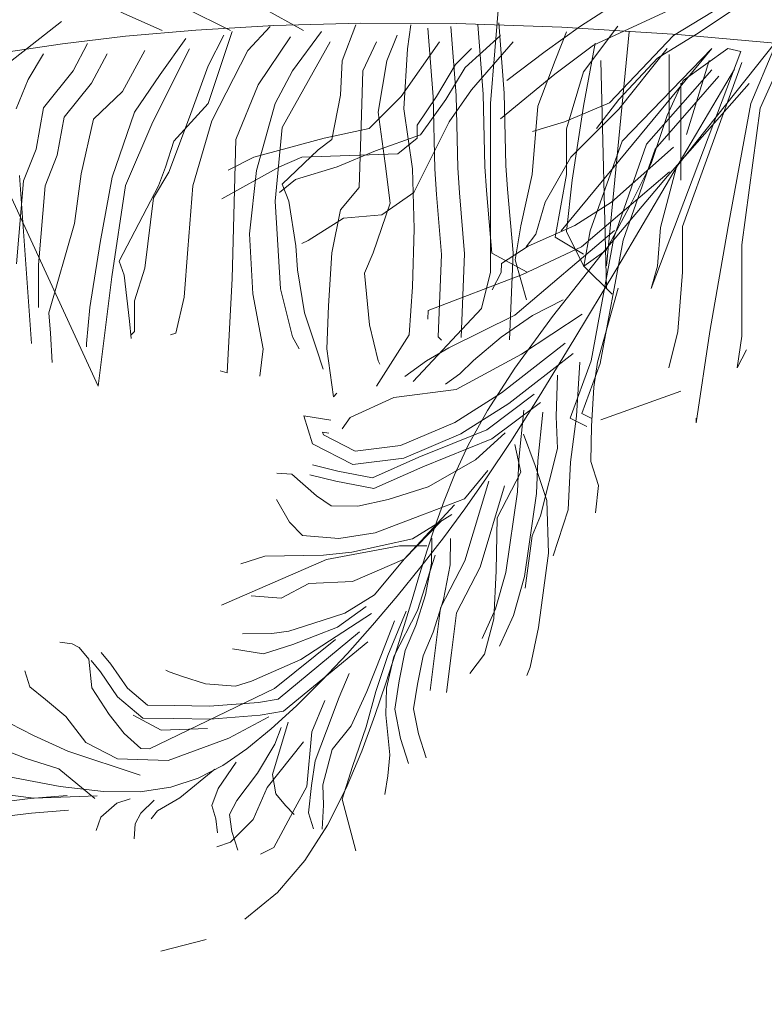
# Model space of a CAD drawing. Units: millimetres. Extents: x 595116 to 630915, y 909473 to 920225.
# Tile 56 of 134: x 629595.727 to 629601.67, y 919288.018 to 919295.882. Entities that reach past the tile are written whole.
import ezdxf

# ---------------------------------------------------------------- set-up
doc = ezdxf.new("R2010")
doc.units = ezdxf.units.MM
doc.layers.add('Dimension', color=3, linetype='Continuous', lineweight=18)
doc.layers.add('L-PLNT', color=85, linetype='Continuous', lineweight=13)
doc.styles.get("Standard").update_dxf_attribs({"font": 'arial.ttf'})
doc.dimstyles.new('ISO-25', dxfattribs={"dimtxt": 9, "dimasz": 6, "dimexe": 1.25, "dimexo": 0.625, "dimtad": 1, "dimlunit": 4, "dimtxsty": 'Standard', "dimcen": 2.5, "dimadec": 0, "dimazin": 0, "dimtfac": 1, "dimtmove": 0, "dimatfit": 3, "dimfxl": 1, "dimarcsym": 0})

# ---------------------------------------------------------------- blocks, each defined once
blk = doc.blocks.new('A$C4FB75ABC')
for p, q in [((2.1065, 2.3741), (2.087, 2.1315)), ((2.5983, 2.3508), (2.4757, 2.2759)), ((1.3881, 2.2867), (1.3008, 2.3255)), ((1.5337, 2.2867), (1.4367, 2.3352)), ((1.6891, 2.2867), (1.6017, 2.3352)), ((2.2781, 2.2963), (2.353, 2.344)), ((2.3054, 2.2555), (2.4825, 2.3372)), ((2.6119, 2.3372), (2.5302, 2.2827)), ((1.1746, 2.3061), (0.9513, 2.1315)), ((1.4598, 2.2878), (1.3106, 2.2744)), ((1.6258, 2.2976), (1.4598, 2.2878)), ((1.5376, 2.2844), (1.4866, 2.1313)), ((1.6179, 2.2954), (1.5705, 2.2443)), ((1.8099, 2.3026), (1.6258, 2.2976)), ((1.7274, 2.2844), (1.6654, 2.2006)), ((1.8004, 2.299), (1.7712, 2.2224)), ((2.0136, 2.3019), (1.8099, 2.3026)), ((1.9171, 2.299), (1.9098, 2.248)), ((1.9536, 2.2917), (1.9646, 2.1459)), ((2.0023, 2.2954), (2.0134, 2.1483)), ((2.2382, 2.2942), (2.0136, 2.3019)), ((2.0597, 2.2997), (2.0708, 2.1511)), ((2.1047, 2.3031), (2.1159, 2.1533)), ((2.2032, 2.2419), (2.2781, 2.2963)), ((2.2482, 2.2839), (2.2239, 2.2232)), ((2.4852, 2.2785), (2.2382, 2.2942)), ((2.3575, 2.296), (2.2846, 2.199)), ((2.3818, 2.2839), (2.3332, 1.7863)), ((1.3106, 2.2744), (1.1767, 2.2586)), ((1.4391, 2.2699), (1.3844, 2.1933)), ((1.5194, 2.2771), (1.4866, 2.2115)), ((1.6617, 2.2735), (1.5924, 2.1714)), ((1.8879, 2.2771), (1.8661, 2.2224)), ((2.1078, 2.2759), (2.0328, 2.2078)), ((2.4757, 2.2759), (2.3394, 2.1329)), ((2.5302, 2.2827), (2.4416, 2.2282)), ((2.7559, 2.2536), (2.4852, 2.2785)), ((1.1767, 2.2586), (1.0564, 2.241)), ((1.23, 2.2589), (1.1992, 2.2008)), ((1.3515, 2.2443), (1.3041, 2.1568)), ((1.4464, 2.2479), (1.3687, 2.0927)), ((1.5705, 2.2443), (1.4939, 2.0948)), ((1.7456, 2.2626), (1.6435, 2.0802)), ((1.8442, 2.2626), (1.815, 2.2006)), ((1.9783, 2.2623), (1.8966, 2.1465)), ((1.9098, 2.248), (1.9025, 2.1203)), ((2.0124, 2.2146), (2.0465, 2.2487)), ((2.135, 2.2623), (2.0465, 2.1602)), ((2.1214, 2.1806), (2.2032, 2.2419)), ((2.2236, 2.1942), (2.3054, 2.2555)), ((2.5574, 2.2487), (2.2372, 1.8605)), ((2.3089, 2.2596), (2.2846, 2.1261)), ((2.462, 2.2487), (2.3599, 2.1193)), ((2.3667, 2.0512), (2.5574, 2.2487)), ((2.428, 1.738), (2.6187, 2.2419)), ((2.6937, 2.2623), (2.4825, 1.9967)), ((2.5915, 2.2487), (2.4961, 2.1806)), ((2.6187, 2.2419), (2.5915, 2.2487)), ((2.6889, 2.2479), (2.6404, 2.1315)), ((1.1363, 2.237), (1.1034, 2.1823)), ((1.2713, 2.237), (1.2384, 2.175)), ((1.7712, 2.2224), (1.7675, 2.1495)), ((1.8661, 2.2224), (1.8478, 2.113)), ((2.2239, 2.2232), (2.1875, 2.1261)), ((2.3211, 2.2232), (2.3332, 1.7378)), ((2.4416, 2.2282), (2.3599, 2.1397)), ((2.4668, 2.2354), (2.4668, 2.0533)), ((2.5518, 2.2232), (2.5032, 2.0655)), ((2.7083, 2.2285), (2.6598, 2.1218)), ((1.1992, 2.2008), (1.1362, 2.1221)), ((1.4866, 2.2115), (1.4464, 2.1021)), ((1.6654, 2.2006), (1.6289, 2.1313)), ((1.815, 2.2006), (1.8113, 2.0838)), ((1.9715, 2.1465), (2.0124, 2.2146)), ((2.0328, 2.2078), (1.992, 2.1397)), ((2.5572, 2.203), (2.4187, 2.0449)), ((2.6056, 2.2048), (2.4676, 1.9701)), ((2.6209, 2.2188), (2.4948, 1.8695)), ((1.1034, 2.1823), (1.0779, 2.1203)), ((1.3844, 2.1933), (1.3297, 2.113)), ((2.1078, 2.0989), (2.2236, 2.1942)), ((2.2846, 2.199), (2.2482, 2.0776)), ((2.5724, 2.1897), (2.4365, 2.0345)), ((2.4961, 2.1806), (2.462, 2.1057)), ((1.2384, 2.175), (1.18, 2.1021)), ((1.5924, 2.1714), (1.5449, 2.0547)), ((2.0465, 2.1602), (1.9988, 2.0921)), ((2.6368, 2.1742), (2.4628, 1.9766)), ((2.4911, 2.1747), (2.4911, 1.9684)), ((1.2522, 1.53), (0.9707, 2.1412)), ((1.3041, 2.1568), (1.2421, 2.0984)), ((1.7675, 2.1495), (1.7493, 2.0547)), ((1.8966, 2.1465), (1.8285, 2.0784)), ((1.9306, 2.0852), (1.9715, 2.1465)), ((1.992, 2.1397), (1.9375, 2.0648)), ((1.9646, 2.1459), (1.9682, 1.9927)), ((2.0134, 2.1483), (2.017, 1.9949)), ((2.0708, 2.1511), (2.0745, 1.9975)), ((2.1159, 2.1533), (2.1196, 1.9995)), ((2.3599, 2.1397), (2.3122, 2.0784)), ((1.1362, 2.1221), (1.1203, 2.0346)), ((1.4866, 2.1313), (1.4136, 2.051)), ((1.6289, 2.1313), (1.5887, 1.989)), ((1.9025, 2.1203), (1.9208, 1.9927)), ((2.087, 2.1315), (2.087, 1.7725)), ((2.1875, 2.1261), (2.1754, 1.9805)), ((2.3394, 2.1329), (2.244, 2.0921)), ((2.3599, 2.1193), (2.2577, 2.0172)), ((2.2846, 2.1261), (2.2604, 1.9684)), ((2.6404, 2.1315), (2.5918, 1.8695)), ((2.6598, 2.1218), (2.6209, 1.8307)), ((1.18, 2.1021), (1.1654, 2.0218)), ((1.2421, 2.0984), (1.2165, 1.9817)), ((1.3297, 2.113), (1.2822, 1.9744)), ((1.4464, 2.1021), (1.4026, 1.9854)), ((1.8478, 2.113), (1.8624, 2.0036)), ((2.462, 2.1057), (2.428, 2.0035)), ((1.3687, 2.0927), (1.3105, 1.9569)), ((1.4939, 2.0948), (1.4537, 1.9562)), ((1.6435, 2.0802), (1.6289, 1.9234)), ((1.8285, 2.0784), (1.7331, 2.058)), ((1.8113, 2.0838), (1.8077, 1.9526)), ((1.9988, 2.0921), (1.9238, 1.9422)), ((1.9306, 2.058), (1.9306, 2.0852)), ((2.244, 2.0921), (2.1759, 2.0716)), ((2.2482, 2.0776), (2.2482, 1.9805)), ((1.5449, 2.0547), (1.5376, 1.7593)), ((1.7331, 2.058), (1.5832, 2.0172)), ((1.7493, 2.0547), (1.7201, 2.0328)), ((1.9375, 2.0648), (1.8421, 2.0308)), ((1.8898, 2.024), (1.9306, 2.058)), ((1.1203, 2.0346), (1.0939, 1.9669)), ((1.4136, 2.051), (1.3953, 1.9963)), ((1.7201, 2.0328), (1.6435, 1.9598)), ((2.2985, 1.8605), (2.3667, 2.0512)), ((2.4756, 2.0387), (2.3438, 1.9217)), ((2.4187, 2.0449), (2.3489, 1.8456)), ((2.4365, 2.0345), (2.3686, 1.8404)), ((1.1654, 2.0218), (1.1399, 1.9562)), ((1.5832, 2.0172), (1.5287, 1.9899)), ((1.6377, 1.9967), (1.6854, 2.0172)), ((1.6854, 2.0172), (1.8898, 2.024)), ((1.8421, 2.0308), (1.7603, 1.9967)), ((2.2577, 2.0172), (2.2032, 1.9218)), ((1.3953, 1.9963), (1.3807, 1.9562)), ((1.5151, 1.9286), (1.6377, 1.9967)), ((1.7603, 1.9967), (1.6718, 1.9695)), ((1.8624, 2.0036), (1.8734, 1.9197)), ((1.9208, 1.9927), (1.9244, 1.865)), ((1.9682, 1.9927), (1.9719, 1.938)), ((2.017, 1.9949), (2.0206, 1.9417)), ((2.0745, 1.9975), (2.0779, 1.946)), ((2.1196, 1.9995), (2.1229, 1.9495)), ((2.428, 2.0035), (2.3871, 1.9218)), ((2.4825, 1.9967), (2.4484, 1.8673)), ((1.0852, 1.9781), (1.1107, 1.6207)), ((1.2165, 1.9817), (1.2019, 1.876)), ((1.2822, 1.9744), (1.2567, 1.8358)), ((1.4026, 1.9854), (1.3698, 1.9307)), ((1.5887, 1.989), (1.5741, 1.8541)), ((1.6718, 1.9695), (1.6377, 1.9422)), ((2.1754, 1.9805), (2.1511, 1.8713)), ((2.2482, 1.9805), (2.2239, 1.847)), ((2.4673, 1.986), (2.2802, 1.8264)), ((2.4628, 1.9766), (2.3249, 1.8127)), ((2.4676, 1.9701), (2.3552, 1.7802)), ((1.0939, 1.9669), (1.0786, 1.7905)), ((1.1399, 1.9562), (1.1253, 1.7884)), ((1.3105, 1.9569), (1.2814, 1.7628)), ((1.3807, 1.9562), (1.2968, 1.7957)), ((1.4537, 1.9562), (1.4428, 1.8213)), ((1.6435, 1.9598), (1.6581, 1.9234)), ((1.8077, 1.9526), (1.7675, 1.9051)), ((2.1229, 1.9495), (2.1345, 1.8136)), ((2.2604, 1.9684), (2.2482, 1.8591)), ((1.3698, 1.9307), (1.3515, 1.7811)), ((1.9238, 1.9422), (1.8557, 1.8946)), ((1.9719, 1.938), (1.9828, 1.8103)), ((2.0206, 1.9417), (2.0317, 1.8114)), ((2.0779, 1.946), (2.0893, 1.8127)), ((1.6289, 1.9234), (1.6398, 1.7374)), ((1.6581, 1.9234), (1.6727, 1.8285)), ((1.8734, 1.9197), (1.8369, 1.814)), ((2.2032, 1.9218), (2.1827, 1.8537)), ((2.3438, 1.9217), (2.2657, 1.8718)), ((2.3871, 1.9218), (2.3326, 1.8197)), ((1.7739, 1.8878), (1.699, 1.8401)), ((1.7675, 1.9051), (1.7493, 1.814)), ((1.8557, 1.8946), (1.7739, 1.8878)), ((1.2019, 1.876), (1.1472, 1.6863)), ((1.9244, 1.865), (1.9208, 1.741)), ((2.1511, 1.8713), (2.1389, 1.7985)), ((2.2657, 1.8718), (2.167, 1.8279)), ((2.4484, 1.8673), (2.4416, 1.7856)), ((2.4948, 1.8695), (2.4948, 1.7725)), ((2.5918, 1.8695), (2.553, 1.6464)), ((1.5741, 1.8541), (1.5814, 1.7264)), ((2.3505, 1.8613), (2.1386, 1.6813)), ((2.1827, 1.8537), (2.1623, 1.8265)), ((2.2239, 1.847), (2.2846, 1.8106)), ((2.2482, 1.8591), (2.2846, 1.7863)), ((2.2849, 1.7856), (2.2985, 1.8605)), ((2.3489, 1.8456), (2.3004, 1.5838)), ((1.2567, 1.8358), (1.2348, 1.6973)), ((1.6727, 1.8285), (1.6763, 1.7775)), ((1.699, 1.8401), (1.6854, 1.8333)), ((2.167, 1.8279), (2.1099, 1.791)), ((2.2802, 1.8264), (2.1549, 1.7678)), ((2.3686, 1.8404), (2.32, 1.5785)), ((2.6209, 1.8307), (2.6209, 1.6367)), ((1.4428, 1.8213), (1.4355, 1.7191)), ((1.7493, 1.814), (1.742, 1.7009)), ((1.8369, 1.814), (1.8186, 1.7702)), ((1.9828, 1.8103), (1.9755, 1.6352)), ((2.0317, 1.8114), (2.0243, 1.6332)), ((2.0893, 1.8127), (2.1647, 1.7725)), ((2.1345, 1.8136), (2.1268, 1.6289)), ((2.3249, 1.8127), (2.2184, 1.678)), ((2.3326, 1.8197), (2.2849, 1.7856)), ((1.1253, 1.7884), (1.1253, 1.7665)), ((1.2968, 1.7957), (1.3078, 1.7665)), ((1.3515, 1.7811), (1.3297, 1.7118)), ((2.1099, 1.791), (2.1096, 1.7722)), ((2.1389, 1.7985), (2.1632, 1.7135)), ((2.2846, 1.7863), (2.3453, 1.7256)), ((2.4416, 1.7856), (2.428, 1.738)), ((1.1253, 1.7665), (1.1253, 1.7301)), ((1.2814, 1.7628), (1.2522, 1.53)), ((1.3078, 1.7665), (1.3187, 1.6681)), ((1.6763, 1.7775), (1.6909, 1.6863)), ((1.8186, 1.7702), (1.8296, 1.6608)), ((2.1549, 1.7678), (1.9538, 1.6913)), ((2.087, 1.7725), (2.0676, 1.6949)), ((2.1096, 1.7722), (2.0903, 1.7347)), ((2.3552, 1.7802), (2.2641, 1.6283)), ((2.4948, 1.7725), (2.485, 1.6464)), ((1.5376, 1.7593), (1.5267, 1.5587)), ((1.9208, 1.741), (1.9135, 1.6389)), ((1.1253, 1.7301), (1.1253, 1.6973)), ((1.4355, 1.7191), (1.4172, 1.6425)), ((1.5814, 1.7264), (1.6033, 1.6097)), ((1.6398, 1.7374), (1.6654, 1.6352)), ((2.3582, 1.7386), (2.3145, 1.5808)), ((1.2348, 1.6973), (1.2275, 1.6207)), ((1.3297, 1.7118), (1.3297, 1.6462)), ((1.742, 1.7009), (1.7383, 1.6097)), ((2.2409, 1.7138), (2.1763, 1.6807)), ((1.1472, 1.6863), (1.1509, 1.6425)), ((1.6909, 1.6863), (1.7164, 1.6097)), ((2.0676, 1.6949), (1.922, 1.5397)), ((1.9538, 1.6913), (1.9536, 1.6725)), ((2.1386, 1.6813), (1.998, 1.6115)), ((2.1763, 1.6807), (2.1096, 1.6345)), ((2.2184, 1.678), (2.1385, 1.568)), ((2.2819, 1.6831), (2.1525, 1.5981)), ((1.3187, 1.6681), (1.3224, 1.6316)), ((1.8296, 1.6608), (1.8478, 1.5842)), ((1.1509, 1.6425), (1.1545, 1.5805)), ((1.3297, 1.6462), (1.3224, 1.6389)), ((1.4172, 1.6425), (1.4063, 1.6389)), ((1.6654, 1.6352), (1.68, 1.6097)), ((1.9135, 1.6389), (1.8444, 1.53)), ((1.9755, 1.6352), (1.9828, 1.628)), ((2.1096, 1.6345), (2.0504, 1.5844)), ((2.485, 1.6464), (2.4656, 1.5688)), ((2.553, 1.6464), (2.5239, 1.4523)), ((2.6209, 1.6367), (2.6112, 1.5688)), ((1.2275, 1.6207), (1.2275, 1.6134)), ((2.2452, 1.6213), (2.1098, 1.5157)), ((2.2641, 1.6283), (2.1904, 1.5079)), ((1.6033, 1.6097), (1.596, 1.5514)), ((1.7164, 1.6097), (1.731, 1.566)), ((1.7383, 1.6097), (1.7529, 1.5076)), ((1.998, 1.6115), (1.9504, 1.5839)), ((2.1525, 1.5981), (2.0137, 1.5227)), ((2.2623, 1.5995), (2.1258, 1.493)), ((2.6112, 1.5688), (2.6307, 1.6076)), ((1.8478, 1.5842), (1.8515, 1.5769)), ((1.9504, 1.5839), (1.9047, 1.5506)), ((2.0504, 1.5844), (2.0217, 1.5565)), ((2.3004, 1.5838), (2.256, 1.4617)), ((2.2767, 1.5813), (2.2695, 1.4664)), ((2.32, 1.5785), (2.2812, 1.4717)), ((2.3145, 1.5808), (2.3062, 1.5281)), ((1.5267, 1.5587), (1.5121, 1.5623)), ((2.0217, 1.5565), (1.9912, 1.5343)), ((2.1385, 1.568), (2.0803, 1.4783)), ((2.2292, 1.5537), (2.2261, 1.4651)), ((1.7529, 1.5076), (1.7602, 1.5149)), ((2.0137, 1.5227), (1.8814, 1.5056)), ((2.1098, 1.5157), (2.0109, 1.453)), ((2.1796, 1.5129), (2.0785, 1.437)), ((2.3062, 1.5281), (2.3013, 1.4452)), ((2.4911, 1.5193), (2.3211, 1.4586)), ((1.8814, 1.5056), (1.7884, 1.4636)), ((2.1258, 1.493), (2.0238, 1.4284)), ((2.1927, 1.4954), (2.0894, 1.4177)), ((2.1904, 1.5079), (2.1298, 1.4122)), ((1.7084, 1.4073), (1.6895, 1.4666)), ((1.6895, 1.4666), (1.747, 1.4576)), ((2.0803, 1.4783), (2.039, 1.4043)), ((2.1578, 1.4791), (2.1468, 1.3743)), ((2.1979, 1.4749), (2.187, 1.3714)), ((2.2812, 1.4717), (2.3006, 1.462)), ((1.7884, 1.4636), (1.7711, 1.4393)), ((2.0109, 1.453), (1.8951, 1.4036)), ((2.2261, 1.4651), (2.2289, 1.3972)), ((2.256, 1.4617), (2.2916, 1.4439)), ((2.2695, 1.4664), (2.2568, 1.3685)), ((2.5239, 1.4523), (2.5239, 1.462)), ((1.7313, 1.4266), (1.7295, 1.4323)), ((1.7295, 1.4323), (1.7427, 1.4302)), ((1.7987, 1.3918), (1.7313, 1.4266)), ((2.0238, 1.4284), (1.9024, 1.3766)), ((2.0785, 1.437), (1.9344, 1.3786)), ((2.1181, 1.4308), (2.055, 1.3732)), ((2.1569, 1.4277), (2.1816, 1.3609)), ((2.3013, 1.4452), (2.3002, 1.3698)), ((1.7936, 1.3632), (1.7084, 1.4073)), ((2.0894, 1.4177), (1.9429, 1.3584)), ((2.039, 1.4043), (2.0098, 1.3416)), ((2.1298, 1.4122), (2.0784, 1.3347)), ((2.1385, 1.406), (2.1509, 1.3473)), ((1.8951, 1.4036), (1.7987, 1.3918)), ((2.2289, 1.3972), (2.1929, 1.2544)), ((1.7623, 1.3489), (1.7078, 1.3628)), ((1.9024, 1.3766), (1.7936, 1.3632)), ((1.9344, 1.3786), (1.8357, 1.3347)), ((2.055, 1.3732), (1.9542, 1.3161)), ((2.1468, 1.3743), (2.1439, 1.3053)), ((2.187, 1.3714), (2.1842, 1.3016)), ((2.2568, 1.3685), (2.2516, 1.2668)), ((2.3002, 1.3698), (2.3165, 1.3187)), ((1.6641, 1.3427), (1.6321, 1.345)), ((1.7163, 1.2967), (1.6641, 1.3427)), ((1.7575, 1.3275), (1.7024, 1.3416)), ((1.8357, 1.3347), (1.7623, 1.3489)), ((1.9429, 1.3584), (1.8383, 1.3119)), ((2.0098, 1.3416), (1.9878, 1.2857)), ((2.0811, 1.3502), (2.0312, 1.2905)), ((2.1509, 1.3473), (2.1005, 1.25)), ((2.1816, 1.3609), (2.2062, 1.287)), ((1.8383, 1.3119), (1.7575, 1.3275)), ((2.0784, 1.3347), (2.0319, 1.2687)), ((2.0829, 1.3276), (2.0324, 1.158)), ((1.9542, 1.3161), (1.869, 1.289)), ((2.1165, 1.3176), (2.065, 1.1449)), ((2.1439, 1.3053), (2.1195, 1.1332)), ((2.1842, 1.3016), (2.1591, 1.1247)), ((2.3165, 1.3187), (2.31, 1.2603)), ((1.6589, 1.2409), (1.6313, 1.2885)), ((1.7481, 1.2755), (1.7163, 1.2967)), ((1.869, 1.289), (1.8046, 1.2748)), ((2.0312, 1.2905), (1.9421, 1.2559)), ((1.9878, 1.2857), (1.9691, 1.2327)), ((2.2062, 1.287), (2.2097, 1.1745)), ((1.8046, 1.2748), (1.7481, 1.2755)), ((2.0103, 1.2776), (1.903, 1.1622)), ((2.0319, 1.2687), (1.9864, 1.2075)), ((2.2516, 1.2668), (2.22, 1.1691)), ((1.6868, 1.2123), (1.6589, 1.2409)), ((1.9421, 1.2559), (1.8416, 1.2177)), ((1.9834, 1.244), (1.903, 1.1622)), ((2.0043, 1.257), (1.9206, 1.2053)), ((2.1005, 1.25), (2.0989, 1.1369)), ((2.1929, 1.2544), (2.1754, 1.2112)), ((1.8416, 1.2177), (1.7641, 1.2056)), ((1.9691, 1.2327), (1.952, 1.1808)), ((1.7641, 1.2056), (1.6868, 1.2123)), ((1.9206, 1.2053), (1.792, 1.1769)), ((1.9864, 1.2075), (1.9386, 1.1458)), ((1.9621, 1.2066), (1.9614, 1.1536)), ((2.0017, 1.2061), (2.001, 1.1495)), ((2.1754, 1.2112), (2.1606, 1.1002)), ((1.792, 1.1769), (1.7315, 1.1702)), ((1.7376, 1.1613), (1.8929, 1.1904)), ((1.8929, 1.1904), (1.9511, 1.1904)), ((1.952, 1.1808), (1.9358, 1.129)), ((2.2097, 1.1745), (2.1886, 1.0162)), ((1.5143, 1.0642), (1.7376, 1.1613)), ((1.607, 1.1681), (1.5558, 1.1518)), ((1.7315, 1.1702), (1.607, 1.1681)), ((1.903, 1.1622), (1.793, 1.1147)), ((1.903, 1.1622), (1.8397, 1.0857)), ((1.9692, 1.1707), (1.9317, 1.0524)), ((1.9614, 1.1536), (1.9482, 1.0859)), ((2.0324, 1.158), (1.9806, 1.0581)), ((1.9386, 1.1458), (1.8882, 1.0835)), ((2.001, 1.1495), (1.9867, 1.0762)), ((2.065, 1.1449), (2.0146, 1.0475)), ((2.0989, 1.1369), (2.0937, 1.0351)), ((2.1195, 1.1332), (2.0972, 1.056)), ((1.793, 1.1147), (1.7005, 1.1103)), ((1.9358, 1.129), (1.9198, 1.076)), ((2.1591, 1.1247), (2.1353, 1.0421)), ((1.7005, 1.1103), (1.6416, 1.079)), ((1.6416, 1.079), (1.5775, 1.0837)), ((1.8397, 1.0857), (1.7769, 1.047)), ((1.8882, 1.0835), (1.8359, 1.0215)), ((1.9198, 1.076), (1.903, 1.0206)), ((1.9482, 1.0859), (1.9278, 1.0204)), ((1.9867, 1.0762), (1.965, 1.0067)), ((1.8224, 1.0615), (1.7614, 1.017)), ((1.9071, 1.0509), (1.8681, 0.9571)), ((1.9317, 1.0524), (1.8813, 0.9551)), ((1.9806, 1.0581), (1.9586, 0.8825)), ((2.0972, 1.056), (2.0692, 0.9929)), ((1.8335, 1.0462), (1.6831, 0.9483)), ((1.7769, 1.047), (1.7087, 1.0253)), ((1.8823, 1.0305), (1.8549, 0.9592)), ((2.0146, 1.0475), (2.004, 0.9628)), ((2.0937, 1.0351), (2.0738, 0.96)), ((2.1353, 1.0421), (2.1061, 0.9765)), ((1.6576, 1.009), (1.6216, 1.0039)), ((1.8084, 1.007), (1.6348, 0.8642)), ((1.7087, 1.0253), (1.6576, 1.009)), ((1.7614, 1.017), (1.6666, 0.9806)), ((1.8359, 1.0215), (1.7823, 0.9612)), ((1.903, 1.0206), (1.8847, 0.9618)), ((1.9278, 1.0204), (1.9055, 0.9679)), ((1.965, 1.0067), (1.9435, 0.9561)), ((2.1886, 1.0162), (2.171, 0.9318)), ((1.1969, 0.9814), (1.1705, 0.9855)), ((1.6216, 1.0039), (1.5594, 1.0028)), ((1.7573, 0.9907), (1.6276, 0.8869)), ((1.8259, 0.9857), (1.6466, 0.8382)), ((1.2119, 0.9737), (1.1969, 0.9814)), ((1.2323, 0.9489), (1.2119, 0.9737)), ((1.6041, 0.9607), (1.5382, 0.9711)), ((1.6666, 0.9806), (1.6041, 0.9607)), ((1.9055, 0.9679), (1.8924, 0.9029)), ((1.239, 0.8884), (1.2323, 0.9489)), ((1.2572, 0.9222), (1.2376, 0.9461)), ((1.2793, 0.9388), (1.2589, 0.9636)), ((1.6831, 0.9483), (1.5787, 0.9026)), ((1.7823, 0.9612), (1.7281, 0.9036)), ((1.8549, 0.9592), (1.8236, 0.8804)), ((1.8681, 0.9571), (1.8425, 0.8802)), ((1.8847, 0.9618), (1.8642, 0.8983)), ((1.8813, 0.9551), (1.8652, 0.8874)), ((1.9435, 0.9561), (1.9314, 0.8959)), ((2.004, 0.9628), (1.9934, 0.8781)), ((2.0738, 0.96), (2.043, 0.9189)), ((1.107, 0.8902), (1.0961, 0.9243)), ((1.2938, 0.8688), (1.2572, 0.9222)), ((1.3144, 0.8874), (1.2793, 0.9388)), ((1.4036, 0.922), (1.3961, 0.9259)), ((1.4317, 0.9122), (1.4036, 0.922)), ((2.171, 0.9318), (2.164, 0.9142)), ((1.4805, 0.8964), (1.4317, 0.9122)), ((1.5787, 0.9026), (1.5446, 0.8918)), ((1.7281, 0.9036), (1.6739, 0.8498)), ((1.7864, 0.9186), (1.765, 0.868)), ((1.8924, 0.9029), (1.8829, 0.8424)), ((1.1405, 0.8634), (1.107, 0.8902)), ((1.2759, 0.8314), (1.239, 0.8884)), ((1.3573, 0.851), (1.3144, 0.8874)), ((1.6276, 0.8869), (1.3617, 0.7585)), ((1.5446, 0.8918), (1.4805, 0.8964)), ((1.8236, 0.8804), (1.7906, 0.8073)), ((1.8425, 0.8802), (1.8226, 0.805)), ((1.8642, 0.8983), (1.8405, 0.829)), ((1.8652, 0.8874), (1.8644, 0.8308)), ((1.9314, 0.8959), (1.9231, 0.8432)), ((1.1834, 0.827), (1.1405, 0.8634)), ((1.347, 0.8236), (1.2938, 0.8688)), ((1.6348, 0.8642), (1.5932, 0.8572)), ((1.7347, 0.8614), (1.7065, 0.7946)), ((1.765, 0.868), (1.7376, 0.7967)), ((1.4139, 0.8502), (1.3573, 0.851)), ((1.4893, 0.8492), (1.4139, 0.8502)), ((1.5932, 0.8572), (1.4893, 0.8492)), ((1.6466, 0.8382), (1.5965, 0.8298)), ((1.6739, 0.8498), (1.6204, 0.8011)), ((1.8829, 0.8424), (1.8952, 0.7804)), ((1.9231, 0.8432), (1.9337, 0.7903)), ((1.1149, 0.7864), (1.04, 0.8252)), ((1.226, 0.7717), (1.1834, 0.827)), ((1.3074, 0.7913), (1.2759, 0.8314)), ((1.3863, 0.7981), (1.3265, 0.8298)), ((1.4135, 0.8227), (1.347, 0.8236)), ((1.4902, 0.8216), (1.4135, 0.8227)), ((1.5965, 0.8298), (1.4902, 0.8216)), ((1.6154, 0.8267), (1.5299, 0.7807)), ((1.8405, 0.829), (1.8129, 0.7535)), ((1.8644, 0.8308), (1.8727, 0.7459)), ((1.4848, 0.8016), (1.3863, 0.7981)), ((1.6204, 0.8011), (1.5682, 0.7585)), ((1.6567, 0.8148), (1.6231, 0.704)), ((1.6415, 0.8037), (1.6278, 0.7681)), ((1.7376, 0.7967), (1.7141, 0.733)), ((1.7906, 0.8073), (1.7502, 0.757)), ((1.8226, 0.805), (1.7931, 0.7206)), ((1.188, 0.7534), (1.1149, 0.7864)), ((1.3428, 0.7588), (1.3074, 0.7913)), ((1.5299, 0.7807), (1.4009, 0.7335)), ((1.7065, 0.7946), (1.696, 0.6785)), ((1.8952, 0.7804), (1.9122, 0.7271)), ((1.9337, 0.7903), (1.9499, 0.7392)), ((1.0992, 0.7376), (1.0204, 0.7689)), ((1.2935, 0.7368), (1.226, 0.7717)), ((1.3617, 0.7585), (1.3428, 0.7588)), ((1.5682, 0.7585), (1.5172, 0.7231)), ((1.6278, 0.7681), (1.5911, 0.7064)), ((1.6891, 0.7732), (1.6114, 0.6762)), ((1.7502, 0.757), (1.7303, 0.6818)), ((1.1687, 0.7159), (1.0992, 0.7376)), ((1.342, 0.7022), (1.188, 0.7534)), ((1.4009, 0.7335), (1.2935, 0.7368)), ((1.8129, 0.7535), (1.7799, 0.6746)), ((1.8727, 0.7459), (1.8683, 0.7007)), ((1.2451, 0.6526), (1.1687, 0.7159)), ((1.5006, 0.7151), (1.4262, 0.6539)), ((1.5172, 0.7231), (1.4647, 0.6957)), ((1.5461, 0.7296), (1.5076, 0.6736)), ((1.7141, 0.733), (1.7058, 0.6803)), ((1.7931, 0.7206), (1.7714, 0.6511)), ((1.1712, 0.6779), (1.0599, 0.6997)), ((1.4647, 0.6957), (1.4072, 0.6768)), ((1.5911, 0.7064), (1.5469, 0.6485)), ((1.6231, 0.704), (1.6301, 0.6625)), ((1.8683, 0.7007), (1.8621, 0.6612)), ((1.2639, 0.6673), (1.1712, 0.6779)), ((1.4072, 0.6768), (1.3414, 0.6671)), ((1.5076, 0.6736), (1.4939, 0.6379)), ((1.6114, 0.6762), (1.5823, 0.6082)), ((1.696, 0.6785), (1.6713, 0.6328)), ((1.7058, 0.6803), (1.6993, 0.6219)), ((1.7303, 0.6818), (1.7316, 0.6384)), ((1.7799, 0.6746), (1.74, 0.5958)), ((1.1074, 0.6526), (1.011, 0.6408)), ((1.1159, 0.6537), (1.0423, 0.6629)), ((1.1867, 0.6591), (1.1074, 0.6526)), ((1.2504, 0.6584), (1.1159, 0.6537)), ((1.3414, 0.6671), (1.2639, 0.6673)), ((1.3206, 0.6516), (1.2921, 0.6426)), ((1.4262, 0.6539), (1.3787, 0.6263)), ((1.6301, 0.6625), (1.6505, 0.6377)), ((1.7714, 0.6511), (1.8, 0.5413)), ((1.2921, 0.6426), (1.2578, 0.6129)), ((1.3714, 0.649), (1.3428, 0.6211)), ((1.4939, 0.6379), (1.5029, 0.6095)), ((1.5469, 0.6485), (1.5314, 0.6186)), ((1.6713, 0.6328), (1.6256, 0.5484)), ((1.6505, 0.6377), (1.6691, 0.6186)), ((1.7316, 0.6384), (1.729, 0.5876)), ((1.1106, 0.6216), (1.016, 0.61)), ((1.1893, 0.628), (1.1106, 0.6216)), ((1.2578, 0.6129), (1.2479, 0.5847)), ((1.3428, 0.6211), (1.3311, 0.5987)), ((1.3787, 0.6263), (1.3652, 0.6095)), ((1.5029, 0.6095), (1.5063, 0.5793)), ((1.5314, 0.6186), (1.5365, 0.5827)), ((1.5823, 0.6082), (1.5337, 0.5597)), ((1.6993, 0.6219), (1.7101, 0.5878)), ((1.3311, 0.5987), (1.3288, 0.5666)), ((1.74, 0.5958), (1.6917, 0.5207)), ((1.5365, 0.5827), (1.5492, 0.5429)), ((1.5337, 0.5597), (1.5046, 0.55)), ((1.6256, 0.5484), (1.5974, 0.5343)), ((1.6917, 0.5207), (1.6336, 0.4527)), ((1.6336, 0.4527), (1.5642, 0.3956)), ((1.4819, 0.3527), (1.3853, 0.3277))]:
    blk.add_line(p, q)
blk = doc.blocks.new('*D210')
at = {"layer": 'Defpoints', "color": 0, "transparency": 16777216}
for p in [(629586.2273, 919310.1229), (629593.9463, 919310.1229), (629586.2273, 919258.6624)]:
    blk.add_point(p, dxfattribs=at)
at = {"layer": 'Dimension', "color": 0, "lineweight": -2, "transparency": 16777216}
for p, q in [((629593.9463, 919310.1229), (629593.9463, 919449.6901)), ((629586.8523, 919310.1229), (629595.1963, 919310.1229)), ((629593.9463, 919264.6624), (629593.9463, 919304.1229)), ((629586.8523, 919258.6624), (629595.1963, 919258.6624))]:
    blk.add_line(p, q, dxfattribs=at)
at = {"layer": 'Dimension', "color": 0, "transparency": 16777216}
for points in [[(629592.9463, 919304.1229), (629594.9463, 919304.1229), (629593.9463, 919310.1229)], [(629592.9463, 919264.6624), (629594.9463, 919264.6624), (629593.9463, 919258.6624)]]:
    blk.add_solid(points, dxfattribs=at)
at = {"layer": 'Dimension', "color": 0, "transparency": 16777216, "insert": (629588.6617, 919382.9065), "char_height": 9, "attachment_point": 5, "rotation": 90}
blk.add_mtext('CANOPY 4\'-3 1/2" TYP.', dxfattribs=at)
blk = doc.blocks.new('*D216')
at = {"layer": 'Defpoints', "color": 0, "transparency": 16777216}
for p in [(629743.5408, 919411.9276), (629505.0408, 919411.8279), (629743.5408, 918832.3776)]:
    blk.add_point(p, dxfattribs=at)
at = {"layer": 'Dimension', "color": 0, "lineweight": -2, "transparency": 16777216}
for p, q in [((629743.5408, 919411.3026), (629743.5408, 918831.1276)), ((629505.0408, 919411.2029), (629505.0408, 918831.1276)), ((629511.0408, 918832.3776), (629737.5408, 918832.3776))]:
    blk.add_line(p, q, dxfattribs=at)
at = {"layer": 'Dimension', "color": 0, "transparency": 16777216}
for points in [[(629511.0408, 918833.3776), (629511.0408, 918831.3776), (629505.0408, 918832.3776)], [(629737.5408, 918833.3776), (629737.5408, 918831.3776), (629743.5408, 918832.3776)]]:
    blk.add_solid(points, dxfattribs=at)
at = {"layer": 'Dimension', "color": 0, "transparency": 16777216, "insert": (629624.2908, 918837.656), "char_height": 9, "attachment_point": 5}
blk.add_mtext('19\'-10 1/2"', dxfattribs=at)

msp = doc.modelspace()

# ---------------------------------------------------------------- block references
at = {"layer": 'L-PLNT', "xscale": 3.753413438031968, "yscale": 3.753413438031968, "zscale": 3.753413438031968}
msp.add_blockref('A$C4FB75ABC', (629591.6528, 919287.2124), dxfattribs=at)

# ---------------------------------------------------------------- dimensions: what is measured, and where the dimension line sits
at = {"layer": 'Dimension'}
dim = msp.add_linear_dim(base=(629593.9463, 919310.1229), p1=(629586.2273, 919258.6624), p2=(629586.2273, 919310.1229), angle=90, text='CANOPY <> TYP.', dimstyle='ISO-25', override={"dimdec": 1, "dimlfac": 1, "dimrnd": 0, "dimzin": 1, "dimdsep": 46, "dimlunit": 4, "dimfrac": 2}, dxfattribs=at)
dim.commit()
dim.dimension.update_dxf_attribs({"geometry": '*D210', "text_midpoint": (629588.6617, 919382.9065)})
dim = msp.add_linear_dim(base=(629743.5408, 918832.3776), p1=(629505.0408, 919411.8279), p2=(629743.5408, 919411.9276), dimstyle='ISO-25', override={"dimdec": 1, "dimlfac": 1, "dimrnd": 0, "dimzin": 1, "dimdsep": 46, "dimlunit": 4, "dimfrac": 2}, dxfattribs=at)
dim.commit()
dim.dimension.update_dxf_attribs({"geometry": '*D216', "text_midpoint": (629624.2908, 918837.656)})

doc.saveas('drawing.dxf')
